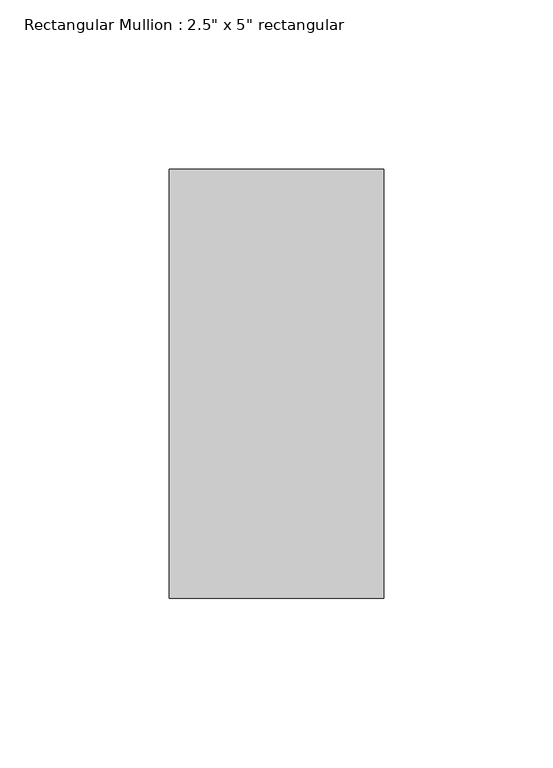
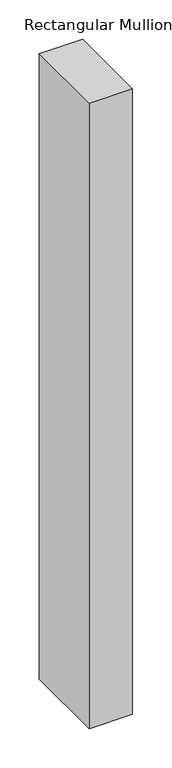
"""IFC4 building model written with IfcOpenShell, lengths in millimetres: member geometry."""

from ifc_helpers import new_model, si_unit, frame, origin, place, context, project, spatial, polyline, outline, extrude, source, transform, mapped, element, save


def member_801a2072(model_context):
    return source(origin(), model_context, "Body", "SweptSolid", [
        extrude(outline(polyline([(0.0, 63.5), (0.0, -63.5), (-63.5, -63.5), (-63.5, 63.5), (0.0, 63.5)])), frame((0.0, 0.0, -971.55), z_axis=(0.0, 0.0, 1.0), x_axis=(1.0, 0.0, 0.0)), (0.0, 0.0, 1.0), 971.55),
    ])


if __name__ == "__main__":
    model = new_model("IFC4")
    model_context = context("Model", 3, world=origin())
    ifc_project = project(units=[si_unit("LENGTHUNIT", "METRE", prefix="MILLI")], contexts=[model_context])
    site = spatial("IfcSite", under=ifc_project)
    building = spatial("IfcBuilding", under=site)
    placement = place(None, origin())
    member_shape = member_801a2072(model_context)
    element("IfcMember", 1, ObjectType="Rectangular Mullion : 2.5\" x 5\" rectangular", at=placement, inside=building, context=model_context, shape_type="MappedRepresentation", body=[
        mapped(member_shape, transform((0.0, 0.0, 0.0), x_axis=(1.0, 0.0, 0.0), y_axis=(0.0, 1.0, 0.0), z_axis=(0.0, 0.0, 1.0))),
    ])
    save(model, "model.ifc")

# Revit data of these elements
# Type "Rectangular Mullion : 2.5\" x 5\" rectangular"
#   built-in parameter 1007304 = 0.416667 (stored number, unit not read)
#   built-in parameter 1007301 = 0.104167 (stored number, unit not read)
#   built-in parameter 1007300 = 0.104167 (stored number, unit not read)
# Element 1 (IfcMember, "Rectangular Mullion : 2.5\" x 5\" rectangular")
#   Materials on its faces: "Aluminum"
# Materials
#   "Aluminum": class "Metal", colour RGB 247 247 247, transparency 0, Description = "Aluminum 6061", Cost = 0
